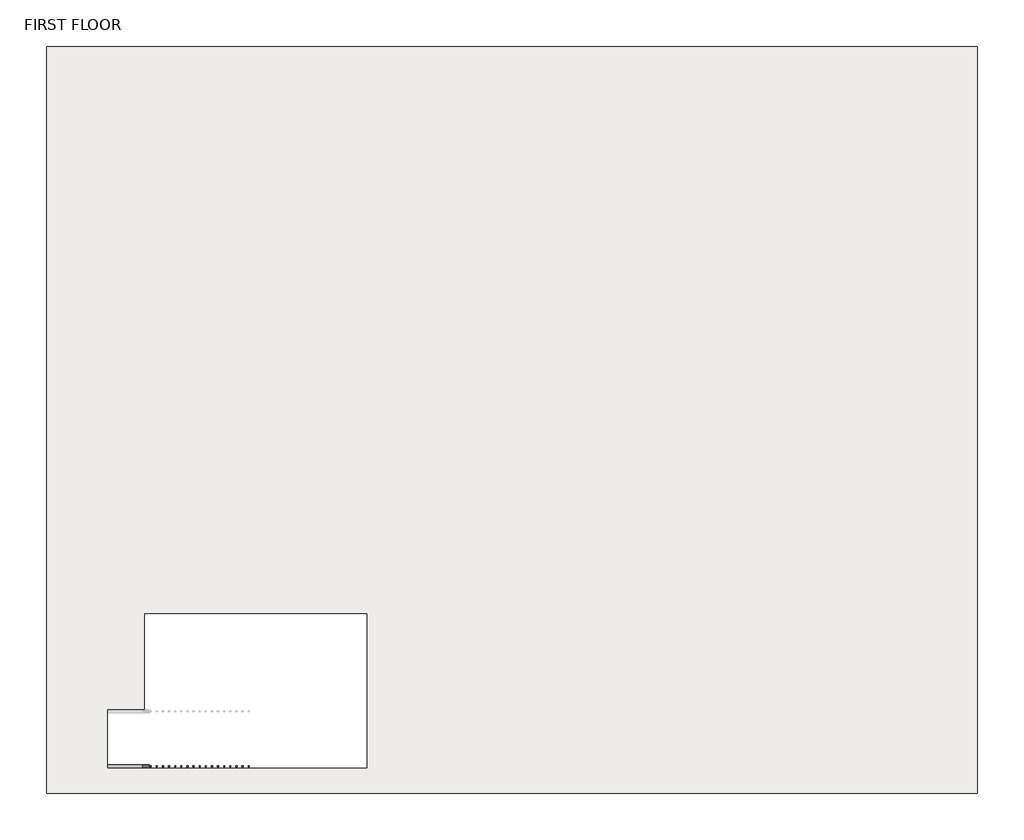
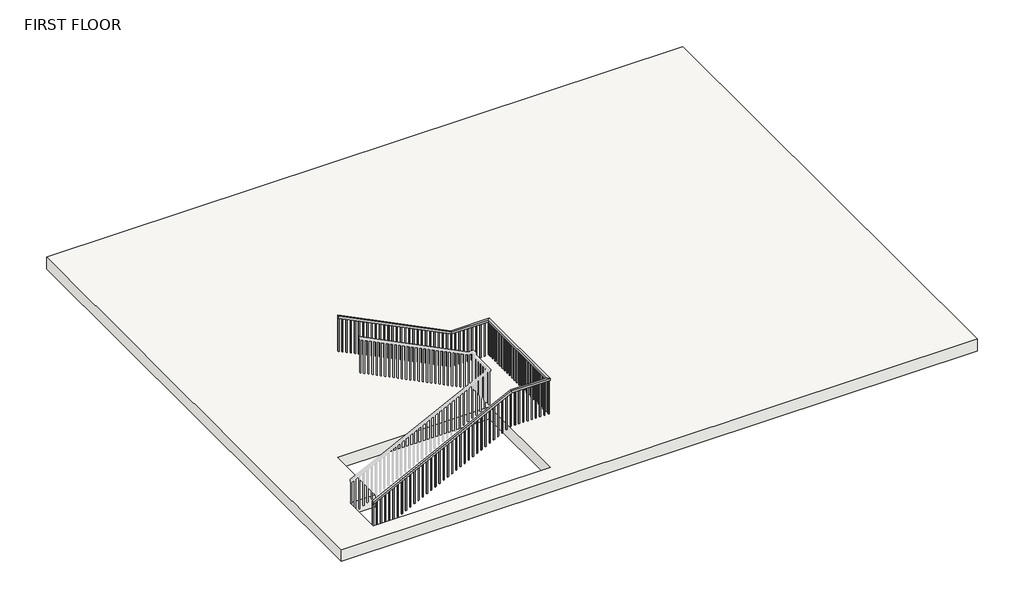
# One storey, part 1 of 2: 1 railing, 1 slab.
"""IFC4 building model written with IfcOpenShell, lengths in millimetres."""

from ifc_helpers import new_model, si_unit, frame, origin, place, context, project, spatial, polyline, outline, extrude, faceted_brep, element, save

model = new_model("IFC4")

# Units and contexts
model_context = context("Model", 3, world=origin())
ifc_project = project(units=[si_unit("LENGTHUNIT", "METRE", prefix="MILLI")], contexts=[model_context])

# Site, building, storey
site = spatial("IfcSite", under=ifc_project)
building = spatial("IfcBuilding", under=site)
storey = spatial("IfcBuildingStorey", under=building, Name="FIRST FLOOR", Elevation=3048.0)

# Railing
placement = place(None, origin())
element("IfcRailing", 1, ObjectType="Handrail - Rectangular", at=placement, inside=storey, context=model_context, shape_type="SolidModel", body=[
    faceted_brep([(-8362.2800418, -5370.1090076, 3962.4), (-8362.2800418, -5370.1090076, 3905.6038734), (-8362.2800418, -5420.9090076, 3905.6038734), (-8362.2800418, -5420.9090076, 3962.4), (-5009.4800418, -5370.1090076, 5638.8), (-4997.4877885, -5370.1090076, 5588.0), (-4997.4877885, -5420.9090076, 5588.0), (-5009.4800418, -5420.9090076, 5638.8), (-4120.4800418, -5370.1090076, 5638.8), (-4120.4800418, -5370.1090076, 5588.0), (-4069.6800418, -5420.9090076, 5588.0), (-4069.6800418, -5420.9090076, 5638.8), (-4120.4800418, -2917.1346494, 5638.8), (-4120.4800418, -2917.1346494, 5588.0), (-4069.6800418, -2866.3346494, 5588.0), (-4069.6800418, -2866.3346494, 5638.8), (-5009.4800418, -2917.1346494, 5638.8), (-5021.472295, -2917.1346494, 5588.0), (-5021.472295, -2866.3346494, 5588.0), (-5009.4800418, -2866.3346494, 5638.8), (-7752.6800418, -2917.1346494, 7010.4), (-7752.6800418, -2866.3346494, 7010.4), (-7752.6800418, -2866.3346494, 6953.6038734), (-7752.6800418, -2917.1346494, 6953.6038734)], [[[0, 1, 2, 3]], [[1, 0, 4, 5]], [[2, 1, 5, 6]], [[3, 2, 6, 7]], [[0, 3, 7, 4]], [[5, 4, 8, 9]], [[6, 5, 9, 10]], [[7, 6, 10, 11]], [[4, 7, 11, 8]], [[9, 8, 12, 13]], [[10, 9, 13, 14]], [[11, 10, 14, 15]], [[8, 11, 15, 12]], [[13, 12, 16, 17]], [[14, 13, 17, 18]], [[15, 14, 18, 19]], [[12, 15, 19, 16]], [[20, 21, 22, 23]], [[17, 16, 20, 23]], [[18, 17, 23, 22]], [[19, 18, 22, 21]], [[16, 19, 21, 20]]]),
    extrude(outline(polyline([(6907.5663734, -7660.6050418), (6049.9625, -7660.6050418), (6040.4375, -7641.5550418), (6898.0413734, -7641.5550418), (6907.5663734, -7660.6050418)])), frame((0.0, -2901.2596494, 0.0), z_axis=(0.0, 1.0, 0.0), x_axis=(0.0, 0.0, 1.0)), (0.0, 0.0, 1.0), 19.05),
    extrude(outline(polyline([(6856.7663734, -7559.0050418), (5999.1625, -7559.0050418), (5989.6375, -7539.9550418), (6847.2413734, -7539.9550418), (6856.7663734, -7559.0050418)])), frame((0.0, -2901.2596494, 0.0), z_axis=(0.0, 1.0, 0.0), x_axis=(0.0, 0.0, 1.0)), (0.0, 0.0, 1.0), 19.05),
    extrude(outline(polyline([(6805.9663734, -7457.4050418), (5948.3625, -7457.4050418), (5938.8375, -7438.3550418), (6796.4413734, -7438.3550418), (6805.9663734, -7457.4050418)])), frame((0.0, -2901.2596494, 0.0), z_axis=(0.0, 1.0, 0.0), x_axis=(0.0, 0.0, 1.0)), (0.0, 0.0, 1.0), 19.05),
    extrude(outline(polyline([(6755.1663734, -7355.8050418), (5897.5625, -7355.8050418), (5888.0375, -7336.7550418), (6745.6413734, -7336.7550418), (6755.1663734, -7355.8050418)])), frame((0.0, -2901.2596494, 0.0), z_axis=(0.0, 1.0, 0.0), x_axis=(0.0, 0.0, 1.0)), (0.0, 0.0, 1.0), 19.05),
    extrude(outline(polyline([(6704.3663734, -7254.2050418), (5846.7625, -7254.2050418), (5837.2375, -7235.1550418), (6694.8413734, -7235.1550418), (6704.3663734, -7254.2050418)])), frame((0.0, -2901.2596494, 0.0), z_axis=(0.0, 1.0, 0.0), x_axis=(0.0, 0.0, 1.0)), (0.0, 0.0, 1.0), 19.05),
    extrude(outline(polyline([(6653.5663734, -7152.6050418), (5795.9625, -7152.6050418), (5786.4375, -7133.5550418), (6644.0413734, -7133.5550418), (6653.5663734, -7152.6050418)])), frame((0.0, -2901.2596494, 0.0), z_axis=(0.0, 1.0, 0.0), x_axis=(0.0, 0.0, 1.0)), (0.0, 0.0, 1.0), 19.05),
    extrude(outline(polyline([(6602.7663734, -7051.0050418), (5745.1625, -7051.0050418), (5735.6375, -7031.9550418), (6593.2413734, -7031.9550418), (6602.7663734, -7051.0050418)])), frame((0.0, -2901.2596494, 0.0), z_axis=(0.0, 1.0, 0.0), x_axis=(0.0, 0.0, 1.0)), (0.0, 0.0, 1.0), 19.05),
    extrude(outline(polyline([(6551.9663734, -6949.4050418), (5694.3625, -6949.4050418), (5684.8375, -6930.3550418), (6542.4413734, -6930.3550418), (6551.9663734, -6949.4050418)])), frame((0.0, -2901.2596494, 0.0), z_axis=(0.0, 1.0, 0.0), x_axis=(0.0, 0.0, 1.0)), (0.0, 0.0, 1.0), 19.05),
    extrude(outline(polyline([(6501.1663734, -6847.8050418), (5643.5625, -6847.8050418), (5634.0375, -6828.7550418), (6491.6413734, -6828.7550418), (6501.1663734, -6847.8050418)])), frame((0.0, -2901.2596494, 0.0), z_axis=(0.0, 1.0, 0.0), x_axis=(0.0, 0.0, 1.0)), (0.0, 0.0, 1.0), 19.05),
    extrude(outline(polyline([(6450.3663734, -6746.2050418), (5592.7625, -6746.2050418), (5583.2375, -6727.1550418), (6440.8413734, -6727.1550418), (6450.3663734, -6746.2050418)])), frame((0.0, -2901.2596494, 0.0), z_axis=(0.0, 1.0, 0.0), x_axis=(0.0, 0.0, 1.0)), (0.0, 0.0, 1.0), 19.05),
    extrude(outline(polyline([(6399.5663734, -6644.6050418), (5541.9625, -6644.6050418), (5532.4375, -6625.5550418), (6390.0413734, -6625.5550418), (6399.5663734, -6644.6050418)])), frame((0.0, -2901.2596494, 0.0), z_axis=(0.0, 1.0, 0.0), x_axis=(0.0, 0.0, 1.0)), (0.0, 0.0, 1.0), 19.05),
    extrude(outline(polyline([(6348.7663734, -6543.0050418), (5491.1625, -6543.0050418), (5481.6375, -6523.9550418), (6339.2413734, -6523.9550418), (6348.7663734, -6543.0050418)])), frame((0.0, -2901.2596494, 0.0), z_axis=(0.0, 1.0, 0.0), x_axis=(0.0, 0.0, 1.0)), (0.0, 0.0, 1.0), 19.05),
    extrude(outline(polyline([(6297.9663734, -6441.4050418), (5440.3625, -6441.4050418), (5430.8375, -6422.3550418), (6288.4413734, -6422.3550418), (6297.9663734, -6441.4050418)])), frame((0.0, -2901.2596494, 0.0), z_axis=(0.0, 1.0, 0.0), x_axis=(0.0, 0.0, 1.0)), (0.0, 0.0, 1.0), 19.05),
    extrude(outline(polyline([(6247.1663734, -6339.8050418), (5389.5625, -6339.8050418), (5380.0375, -6320.7550418), (6237.6413734, -6320.7550418), (6247.1663734, -6339.8050418)])), frame((0.0, -2901.2596494, 0.0), z_axis=(0.0, 1.0, 0.0), x_axis=(0.0, 0.0, 1.0)), (0.0, 0.0, 1.0), 19.05),
    extrude(outline(polyline([(6196.3663734, -6238.2050418), (5338.7625, -6238.2050418), (5329.2375, -6219.1550418), (6186.8413734, -6219.1550418), (6196.3663734, -6238.2050418)])), frame((0.0, -2901.2596494, 0.0), z_axis=(0.0, 1.0, 0.0), x_axis=(0.0, 0.0, 1.0)), (0.0, 0.0, 1.0), 19.05),
    extrude(outline(polyline([(6145.5663734, -6136.6050418), (5287.9625, -6136.6050418), (5278.4375, -6117.5550418), (6136.0413734, -6117.5550418), (6145.5663734, -6136.6050418)])), frame((0.0, -2901.2596494, 0.0), z_axis=(0.0, 1.0, 0.0), x_axis=(0.0, 0.0, 1.0)), (0.0, 0.0, 1.0), 19.05),
    extrude(outline(polyline([(6094.7663734, -6035.0050418), (5237.1625, -6035.0050418), (5227.6375, -6015.9550418), (6085.2413734, -6015.9550418), (6094.7663734, -6035.0050418)])), frame((0.0, -2901.2596494, 0.0), z_axis=(0.0, 1.0, 0.0), x_axis=(0.0, 0.0, 1.0)), (0.0, 0.0, 1.0), 19.05),
    extrude(outline(polyline([(6043.9663734, -5933.4050418), (5186.3625, -5933.4050418), (5176.8375, -5914.3550418), (6034.4413734, -5914.3550418), (6043.9663734, -5933.4050418)])), frame((0.0, -2901.2596494, 0.0), z_axis=(0.0, 1.0, 0.0), x_axis=(0.0, 0.0, 1.0)), (0.0, 0.0, 1.0), 19.05),
    extrude(outline(polyline([(5993.1663734, -5831.8050418), (5135.5625, -5831.8050418), (5126.0375, -5812.7550418), (5983.6413734, -5812.7550418), (5993.1663734, -5831.8050418)])), frame((0.0, -2901.2596494, 0.0), z_axis=(0.0, 1.0, 0.0), x_axis=(0.0, 0.0, 1.0)), (0.0, 0.0, 1.0), 19.05),
    extrude(outline(polyline([(5942.3663734, -5730.2050418), (5084.7625, -5730.2050418), (5075.2375, -5711.1550418), (5932.8413734, -5711.1550418), (5942.3663734, -5730.2050418)])), frame((0.0, -2901.2596494, 0.0), z_axis=(0.0, 1.0, 0.0), x_axis=(0.0, 0.0, 1.0)), (0.0, 0.0, 1.0), 19.05),
    extrude(outline(polyline([(5891.5663734, -5628.6050418), (5033.9625, -5628.6050418), (5024.4375, -5609.5550418), (5882.0413734, -5609.5550418), (5891.5663734, -5628.6050418)])), frame((0.0, -2901.2596494, 0.0), z_axis=(0.0, 1.0, 0.0), x_axis=(0.0, 0.0, 1.0)), (0.0, 0.0, 1.0), 19.05),
    extrude(outline(polyline([(5840.7663734, -5527.0050418), (4983.1625, -5527.0050418), (4973.6375, -5507.9550418), (5831.2413734, -5507.9550418), (5840.7663734, -5527.0050418)])), frame((0.0, -2901.2596494, 0.0), z_axis=(0.0, 1.0, 0.0), x_axis=(0.0, 0.0, 1.0)), (0.0, 0.0, 1.0), 19.05),
    extrude(outline(polyline([(5789.9663734, -5425.4050418), (4932.3625, -5425.4050418), (4922.8375, -5406.3550418), (5780.4413734, -5406.3550418), (5789.9663734, -5425.4050418)])), frame((0.0, -2901.2596494, 0.0), z_axis=(0.0, 1.0, 0.0), x_axis=(0.0, 0.0, 1.0)), (0.0, 0.0, 1.0), 19.05),
    extrude(outline(polyline([(5739.1663734, -5323.8050418), (4881.5625, -5323.8050418), (4872.0375, -5304.7550418), (5729.6413734, -5304.7550418), (5739.1663734, -5323.8050418)])), frame((0.0, -2901.2596494, 0.0), z_axis=(0.0, 1.0, 0.0), x_axis=(0.0, 0.0, 1.0)), (0.0, 0.0, 1.0), 19.05),
    extrude(outline(polyline([(5688.3663734, -5222.2050418), (4830.7625, -5222.2050418), (4821.2375, -5203.1550418), (5678.8413734, -5203.1550418), (5688.3663734, -5222.2050418)])), frame((0.0, -2901.2596494, 0.0), z_axis=(0.0, 1.0, 0.0), x_axis=(0.0, 0.0, 1.0)), (0.0, 0.0, 1.0), 19.05),
    extrude(outline(polyline([(5637.5663734, -5120.6050418), (4779.9625, -5120.6050418), (4770.4375, -5101.5550418), (5628.0413734, -5101.5550418), (5637.5663734, -5120.6050418)])), frame((0.0, -2901.2596494, 0.0), z_axis=(0.0, 1.0, 0.0), x_axis=(0.0, 0.0, 1.0)), (0.0, 0.0, 1.0), 19.05),
    extrude(outline(polyline([(-4898.3550418, -2901.2596494), (-4917.4050418, -2901.2596494), (-4917.4050418, -2882.2096494), (-4898.3550418, -2882.2096494), (-4898.3550418, -2901.2596494)])), frame((0.0, 0.0, 4724.4), z_axis=(0.0, 0.0, 1.0), x_axis=(1.0, 0.0, 0.0)), (0.0, 0.0, 1.0), 863.6),
    extrude(outline(polyline([(-4796.7550418, -2901.2596494), (-4815.8050418, -2901.2596494), (-4815.8050418, -2882.2096494), (-4796.7550418, -2882.2096494), (-4796.7550418, -2901.2596494)])), frame((0.0, 0.0, 4724.4), z_axis=(0.0, 0.0, 1.0), x_axis=(1.0, 0.0, 0.0)), (0.0, 0.0, 1.0), 863.6),
    extrude(outline(polyline([(-4695.1550418, -2901.2596494), (-4714.2050418, -2901.2596494), (-4714.2050418, -2882.2096494), (-4695.1550418, -2882.2096494), (-4695.1550418, -2901.2596494)])), frame((0.0, 0.0, 4724.4), z_axis=(0.0, 0.0, 1.0), x_axis=(1.0, 0.0, 0.0)), (0.0, 0.0, 1.0), 863.6),
    extrude(outline(polyline([(-4593.5550418, -2901.2596494), (-4612.6050418, -2901.2596494), (-4612.6050418, -2882.2096494), (-4593.5550418, -2882.2096494), (-4593.5550418, -2901.2596494)])), frame((0.0, 0.0, 4724.4), z_axis=(0.0, 0.0, 1.0), x_axis=(1.0, 0.0, 0.0)), (0.0, 0.0, 1.0), 863.6),
    extrude(outline(polyline([(-4491.9550418, -2901.2596494), (-4511.0050418, -2901.2596494), (-4511.0050418, -2882.2096494), (-4491.9550418, -2882.2096494), (-4491.9550418, -2901.2596494)])), frame((0.0, 0.0, 4724.4), z_axis=(0.0, 0.0, 1.0), x_axis=(1.0, 0.0, 0.0)), (0.0, 0.0, 1.0), 863.6),
    extrude(outline(polyline([(-4390.3550418, -2901.2596494), (-4409.4050418, -2901.2596494), (-4409.4050418, -2882.2096494), (-4390.3550418, -2882.2096494), (-4390.3550418, -2901.2596494)])), frame((0.0, 0.0, 4724.4), z_axis=(0.0, 0.0, 1.0), x_axis=(1.0, 0.0, 0.0)), (0.0, 0.0, 1.0), 863.6),
    extrude(outline(polyline([(-4288.7550418, -2901.2596494), (-4307.8050418, -2901.2596494), (-4307.8050418, -2882.2096494), (-4288.7550418, -2882.2096494), (-4288.7550418, -2901.2596494)])), frame((0.0, 0.0, 4724.4), z_axis=(0.0, 0.0, 1.0), x_axis=(1.0, 0.0, 0.0)), (0.0, 0.0, 1.0), 863.6),
    extrude(outline(polyline([(-4187.1550418, -2901.2596494), (-4206.2050418, -2901.2596494), (-4206.2050418, -2882.2096494), (-4187.1550418, -2882.2096494), (-4187.1550418, -2901.2596494)])), frame((0.0, 0.0, 4724.4), z_axis=(0.0, 0.0, 1.0), x_axis=(1.0, 0.0, 0.0)), (0.0, 0.0, 1.0), 863.6),
    extrude(outline(polyline([(-4104.6050418, -2966.6340076), (-4104.6050418, -2947.5840076), (-4085.5550418, -2947.5840076), (-4085.5550418, -2966.6340076), (-4104.6050418, -2966.6340076)])), frame((0.0, 0.0, 4724.4), z_axis=(0.0, 0.0, 1.0), x_axis=(1.0, 0.0, 0.0)), (0.0, 0.0, 1.0), 863.6),
    extrude(outline(polyline([(-4104.6050418, -3068.2340076), (-4104.6050418, -3049.1840076), (-4085.5550418, -3049.1840076), (-4085.5550418, -3068.2340076), (-4104.6050418, -3068.2340076)])), frame((0.0, 0.0, 4724.4), z_axis=(0.0, 0.0, 1.0), x_axis=(1.0, 0.0, 0.0)), (0.0, 0.0, 1.0), 863.6),
    extrude(outline(polyline([(-4104.6050418, -3169.8340076), (-4104.6050418, -3150.7840076), (-4085.5550418, -3150.7840076), (-4085.5550418, -3169.8340076), (-4104.6050418, -3169.8340076)])), frame((0.0, 0.0, 4724.4), z_axis=(0.0, 0.0, 1.0), x_axis=(1.0, 0.0, 0.0)), (0.0, 0.0, 1.0), 863.6),
    extrude(outline(polyline([(-4104.6050418, -3271.4340076), (-4104.6050418, -3252.3840076), (-4085.5550418, -3252.3840076), (-4085.5550418, -3271.4340076), (-4104.6050418, -3271.4340076)])), frame((0.0, 0.0, 4724.4), z_axis=(0.0, 0.0, 1.0), x_axis=(1.0, 0.0, 0.0)), (0.0, 0.0, 1.0), 863.6),
    extrude(outline(polyline([(-4104.6050418, -3373.0340076), (-4104.6050418, -3353.9840076), (-4085.5550418, -3353.9840076), (-4085.5550418, -3373.0340076), (-4104.6050418, -3373.0340076)])), frame((0.0, 0.0, 4724.4), z_axis=(0.0, 0.0, 1.0), x_axis=(1.0, 0.0, 0.0)), (0.0, 0.0, 1.0), 863.6),
    extrude(outline(polyline([(-4104.6050418, -3474.6340076), (-4104.6050418, -3455.5840076), (-4085.5550418, -3455.5840076), (-4085.5550418, -3474.6340076), (-4104.6050418, -3474.6340076)])), frame((0.0, 0.0, 4724.4), z_axis=(0.0, 0.0, 1.0), x_axis=(1.0, 0.0, 0.0)), (0.0, 0.0, 1.0), 863.6),
    extrude(outline(polyline([(-4104.6050418, -3576.2340076), (-4104.6050418, -3557.1840076), (-4085.5550418, -3557.1840076), (-4085.5550418, -3576.2340076), (-4104.6050418, -3576.2340076)])), frame((0.0, 0.0, 4724.4), z_axis=(0.0, 0.0, 1.0), x_axis=(1.0, 0.0, 0.0)), (0.0, 0.0, 1.0), 863.6),
    extrude(outline(polyline([(-4104.6050418, -3677.8340076), (-4104.6050418, -3658.7840076), (-4085.5550418, -3658.7840076), (-4085.5550418, -3677.8340076), (-4104.6050418, -3677.8340076)])), frame((0.0, 0.0, 4724.4), z_axis=(0.0, 0.0, 1.0), x_axis=(1.0, 0.0, 0.0)), (0.0, 0.0, 1.0), 863.6),
    extrude(outline(polyline([(-4104.6050418, -3779.4340076), (-4104.6050418, -3760.3840076), (-4085.5550418, -3760.3840076), (-4085.5550418, -3779.4340076), (-4104.6050418, -3779.4340076)])), frame((0.0, 0.0, 4724.4), z_axis=(0.0, 0.0, 1.0), x_axis=(1.0, 0.0, 0.0)), (0.0, 0.0, 1.0), 863.6),
    extrude(outline(polyline([(-4104.6050418, -3881.0340076), (-4104.6050418, -3861.9840076), (-4085.5550418, -3861.9840076), (-4085.5550418, -3881.0340076), (-4104.6050418, -3881.0340076)])), frame((0.0, 0.0, 4724.4), z_axis=(0.0, 0.0, 1.0), x_axis=(1.0, 0.0, 0.0)), (0.0, 0.0, 1.0), 863.6),
    extrude(outline(polyline([(-4104.6050418, -3982.6340076), (-4104.6050418, -3963.5840076), (-4085.5550418, -3963.5840076), (-4085.5550418, -3982.6340076), (-4104.6050418, -3982.6340076)])), frame((0.0, 0.0, 4724.4), z_axis=(0.0, 0.0, 1.0), x_axis=(1.0, 0.0, 0.0)), (0.0, 0.0, 1.0), 863.6),
    extrude(outline(polyline([(-4104.6050418, -4084.2340076), (-4104.6050418, -4065.1840076), (-4085.5550418, -4065.1840076), (-4085.5550418, -4084.2340076), (-4104.6050418, -4084.2340076)])), frame((0.0, 0.0, 4724.4), z_axis=(0.0, 0.0, 1.0), x_axis=(1.0, 0.0, 0.0)), (0.0, 0.0, 1.0), 863.6),
    extrude(outline(polyline([(-4104.6050418, -4185.8340076), (-4104.6050418, -4166.7840076), (-4085.5550418, -4166.7840076), (-4085.5550418, -4185.8340076), (-4104.6050418, -4185.8340076)])), frame((0.0, 0.0, 4724.4), z_axis=(0.0, 0.0, 1.0), x_axis=(1.0, 0.0, 0.0)), (0.0, 0.0, 1.0), 863.6),
    extrude(outline(polyline([(-4104.6050418, -4287.4340076), (-4104.6050418, -4268.3840076), (-4085.5550418, -4268.3840076), (-4085.5550418, -4287.4340076), (-4104.6050418, -4287.4340076)])), frame((0.0, 0.0, 4724.4), z_axis=(0.0, 0.0, 1.0), x_axis=(1.0, 0.0, 0.0)), (0.0, 0.0, 1.0), 863.6),
    extrude(outline(polyline([(-4104.6050418, -4389.0340076), (-4104.6050418, -4369.9840076), (-4085.5550418, -4369.9840076), (-4085.5550418, -4389.0340076), (-4104.6050418, -4389.0340076)])), frame((0.0, 0.0, 4724.4), z_axis=(0.0, 0.0, 1.0), x_axis=(1.0, 0.0, 0.0)), (0.0, 0.0, 1.0), 863.6),
    extrude(outline(polyline([(-4104.6050418, -4490.6340076), (-4104.6050418, -4471.5840076), (-4085.5550418, -4471.5840076), (-4085.5550418, -4490.6340076), (-4104.6050418, -4490.6340076)])), frame((0.0, 0.0, 4724.4), z_axis=(0.0, 0.0, 1.0), x_axis=(1.0, 0.0, 0.0)), (0.0, 0.0, 1.0), 863.6),
    extrude(outline(polyline([(-4104.6050418, -4592.2340076), (-4104.6050418, -4573.1840076), (-4085.5550418, -4573.1840076), (-4085.5550418, -4592.2340076), (-4104.6050418, -4592.2340076)])), frame((0.0, 0.0, 4724.4), z_axis=(0.0, 0.0, 1.0), x_axis=(1.0, 0.0, 0.0)), (0.0, 0.0, 1.0), 863.6),
    extrude(outline(polyline([(-4104.6050418, -4693.8340076), (-4104.6050418, -4674.7840076), (-4085.5550418, -4674.7840076), (-4085.5550418, -4693.8340076), (-4104.6050418, -4693.8340076)])), frame((0.0, 0.0, 4724.4), z_axis=(0.0, 0.0, 1.0), x_axis=(1.0, 0.0, 0.0)), (0.0, 0.0, 1.0), 863.6),
    extrude(outline(polyline([(-4104.6050418, -4795.4340076), (-4104.6050418, -4776.3840076), (-4085.5550418, -4776.3840076), (-4085.5550418, -4795.4340076), (-4104.6050418, -4795.4340076)])), frame((0.0, 0.0, 4724.4), z_axis=(0.0, 0.0, 1.0), x_axis=(1.0, 0.0, 0.0)), (0.0, 0.0, 1.0), 863.6),
    extrude(outline(polyline([(-4104.6050418, -4897.0340076), (-4104.6050418, -4877.9840076), (-4085.5550418, -4877.9840076), (-4085.5550418, -4897.0340076), (-4104.6050418, -4897.0340076)])), frame((0.0, 0.0, 4724.4), z_axis=(0.0, 0.0, 1.0), x_axis=(1.0, 0.0, 0.0)), (0.0, 0.0, 1.0), 863.6),
    extrude(outline(polyline([(-4104.6050418, -4998.6340076), (-4104.6050418, -4979.5840076), (-4085.5550418, -4979.5840076), (-4085.5550418, -4998.6340076), (-4104.6050418, -4998.6340076)])), frame((0.0, 0.0, 4724.4), z_axis=(0.0, 0.0, 1.0), x_axis=(1.0, 0.0, 0.0)), (0.0, 0.0, 1.0), 863.6),
    extrude(outline(polyline([(-4104.6050418, -5100.2340076), (-4104.6050418, -5081.1840076), (-4085.5550418, -5081.1840076), (-4085.5550418, -5100.2340076), (-4104.6050418, -5100.2340076)])), frame((0.0, 0.0, 4724.4), z_axis=(0.0, 0.0, 1.0), x_axis=(1.0, 0.0, 0.0)), (0.0, 0.0, 1.0), 863.6),
    extrude(outline(polyline([(-4104.6050418, -5201.8340076), (-4104.6050418, -5182.7840076), (-4085.5550418, -5182.7840076), (-4085.5550418, -5201.8340076), (-4104.6050418, -5201.8340076)])), frame((0.0, 0.0, 4724.4), z_axis=(0.0, 0.0, 1.0), x_axis=(1.0, 0.0, 0.0)), (0.0, 0.0, 1.0), 863.6),
    extrude(outline(polyline([(-4104.6050418, -5303.4340076), (-4104.6050418, -5284.3840076), (-4085.5550418, -5284.3840076), (-4085.5550418, -5303.4340076), (-4104.6050418, -5303.4340076)])), frame((0.0, 0.0, 4724.4), z_axis=(0.0, 0.0, 1.0), x_axis=(1.0, 0.0, 0.0)), (0.0, 0.0, 1.0), 863.6),
    extrude(outline(polyline([(-4206.2050418, -5385.9840076), (-4187.1550418, -5385.9840076), (-4187.1550418, -5405.0340076), (-4206.2050418, -5405.0340076), (-4206.2050418, -5385.9840076)])), frame((0.0, 0.0, 4724.4), z_axis=(0.0, 0.0, 1.0), x_axis=(1.0, 0.0, 0.0)), (0.0, 0.0, 1.0), 863.6),
    extrude(outline(polyline([(-4307.8050418, -5385.9840076), (-4288.7550418, -5385.9840076), (-4288.7550418, -5405.0340076), (-4307.8050418, -5405.0340076), (-4307.8050418, -5385.9840076)])), frame((0.0, 0.0, 4724.4), z_axis=(0.0, 0.0, 1.0), x_axis=(1.0, 0.0, 0.0)), (0.0, 0.0, 1.0), 863.6),
    extrude(outline(polyline([(-4409.4050418, -5385.9840076), (-4390.3550418, -5385.9840076), (-4390.3550418, -5405.0340076), (-4409.4050418, -5405.0340076), (-4409.4050418, -5385.9840076)])), frame((0.0, 0.0, 4724.4), z_axis=(0.0, 0.0, 1.0), x_axis=(1.0, 0.0, 0.0)), (0.0, 0.0, 1.0), 863.6),
    extrude(outline(polyline([(-4511.0050418, -5385.9840076), (-4491.9550418, -5385.9840076), (-4491.9550418, -5405.0340076), (-4511.0050418, -5405.0340076), (-4511.0050418, -5385.9840076)])), frame((0.0, 0.0, 4724.4), z_axis=(0.0, 0.0, 1.0), x_axis=(1.0, 0.0, 0.0)), (0.0, 0.0, 1.0), 863.6),
    extrude(outline(polyline([(-4612.6050418, -5385.9840076), (-4593.5550418, -5385.9840076), (-4593.5550418, -5405.0340076), (-4612.6050418, -5405.0340076), (-4612.6050418, -5385.9840076)])), frame((0.0, 0.0, 4724.4), z_axis=(0.0, 0.0, 1.0), x_axis=(1.0, 0.0, 0.0)), (0.0, 0.0, 1.0), 863.6),
    extrude(outline(polyline([(-4714.2050418, -5385.9840076), (-4695.1550418, -5385.9840076), (-4695.1550418, -5405.0340076), (-4714.2050418, -5405.0340076), (-4714.2050418, -5385.9840076)])), frame((0.0, 0.0, 4724.4), z_axis=(0.0, 0.0, 1.0), x_axis=(1.0, 0.0, 0.0)), (0.0, 0.0, 1.0), 863.6),
    extrude(outline(polyline([(-4815.8050418, -5385.9840076), (-4796.7550418, -5385.9840076), (-4796.7550418, -5405.0340076), (-4815.8050418, -5405.0340076), (-4815.8050418, -5385.9840076)])), frame((0.0, 0.0, 4724.4), z_axis=(0.0, 0.0, 1.0), x_axis=(1.0, 0.0, 0.0)), (0.0, 0.0, 1.0), 863.6),
    extrude(outline(polyline([(-4917.4050418, -5385.9840076), (-4898.3550418, -5385.9840076), (-4898.3550418, -5405.0340076), (-4917.4050418, -5405.0340076), (-4917.4050418, -5385.9840076)])), frame((0.0, 0.0, 4724.4), z_axis=(0.0, 0.0, 1.0), x_axis=(1.0, 0.0, 0.0)), (0.0, 0.0, 1.0), 863.6),
    extrude(outline(polyline([(5526.4413734, -5120.6050418), (4668.8375, -5120.6050418), (4678.3625, -5101.5550418), (5535.9663734, -5101.5550418), (5526.4413734, -5120.6050418)])), frame((0.0, -5405.0340076, 0.0), z_axis=(0.0, 1.0, 0.0), x_axis=(0.0, 0.0, 1.0)), (0.0, 0.0, 1.0), 19.05),
    extrude(outline(polyline([(5475.6413734, -5222.2050418), (4618.0375, -5222.2050418), (4627.5625, -5203.1550418), (5485.1663734, -5203.1550418), (5475.6413734, -5222.2050418)])), frame((0.0, -5405.0340076, 0.0), z_axis=(0.0, 1.0, 0.0), x_axis=(0.0, 0.0, 1.0)), (0.0, 0.0, 1.0), 19.05),
    extrude(outline(polyline([(5424.8413734, -5323.8050418), (4567.2375, -5323.8050418), (4576.7625, -5304.7550418), (5434.3663734, -5304.7550418), (5424.8413734, -5323.8050418)])), frame((0.0, -5405.0340076, 0.0), z_axis=(0.0, 1.0, 0.0), x_axis=(0.0, 0.0, 1.0)), (0.0, 0.0, 1.0), 19.05),
    extrude(outline(polyline([(5374.0413734, -5425.4050418), (4516.4375, -5425.4050418), (4525.9625, -5406.3550418), (5383.5663734, -5406.3550418), (5374.0413734, -5425.4050418)])), frame((0.0, -5405.0340076, 0.0), z_axis=(0.0, 1.0, 0.0), x_axis=(0.0, 0.0, 1.0)), (0.0, 0.0, 1.0), 19.05),
    extrude(outline(polyline([(5323.2413734, -5527.0050418), (4465.6375, -5527.0050418), (4475.1625, -5507.9550418), (5332.7663734, -5507.9550418), (5323.2413734, -5527.0050418)])), frame((0.0, -5405.0340076, 0.0), z_axis=(0.0, 1.0, 0.0), x_axis=(0.0, 0.0, 1.0)), (0.0, 0.0, 1.0), 19.05),
    extrude(outline(polyline([(5272.4413734, -5628.6050418), (4414.8375, -5628.6050418), (4424.3625, -5609.5550418), (5281.9663734, -5609.5550418), (5272.4413734, -5628.6050418)])), frame((0.0, -5405.0340076, 0.0), z_axis=(0.0, 1.0, 0.0), x_axis=(0.0, 0.0, 1.0)), (0.0, 0.0, 1.0), 19.05),
    extrude(outline(polyline([(5221.6413734, -5730.2050418), (4364.0375, -5730.2050418), (4373.5625, -5711.1550418), (5231.1663734, -5711.1550418), (5221.6413734, -5730.2050418)])), frame((0.0, -5405.0340076, 0.0), z_axis=(0.0, 1.0, 0.0), x_axis=(0.0, 0.0, 1.0)), (0.0, 0.0, 1.0), 19.05),
    extrude(outline(polyline([(5170.8413734, -5831.8050418), (4313.2375, -5831.8050418), (4322.7625, -5812.7550418), (5180.3663734, -5812.7550418), (5170.8413734, -5831.8050418)])), frame((0.0, -5405.0340076, 0.0), z_axis=(0.0, 1.0, 0.0), x_axis=(0.0, 0.0, 1.0)), (0.0, 0.0, 1.0), 19.05),
    extrude(outline(polyline([(5120.0413734, -5933.4050418), (4262.4375, -5933.4050418), (4271.9625, -5914.3550418), (5129.5663734, -5914.3550418), (5120.0413734, -5933.4050418)])), frame((0.0, -5405.0340076, 0.0), z_axis=(0.0, 1.0, 0.0), x_axis=(0.0, 0.0, 1.0)), (0.0, 0.0, 1.0), 19.05),
    extrude(outline(polyline([(5069.2413734, -6035.0050418), (4211.6375, -6035.0050418), (4221.1625, -6015.9550418), (5078.7663734, -6015.9550418), (5069.2413734, -6035.0050418)])), frame((0.0, -5405.0340076, 0.0), z_axis=(0.0, 1.0, 0.0), x_axis=(0.0, 0.0, 1.0)), (0.0, 0.0, 1.0), 19.05),
    extrude(outline(polyline([(5018.4413734, -6136.6050418), (4160.8375, -6136.6050418), (4170.3625, -6117.5550418), (5027.9663734, -6117.5550418), (5018.4413734, -6136.6050418)])), frame((0.0, -5405.0340076, 0.0), z_axis=(0.0, 1.0, 0.0), x_axis=(0.0, 0.0, 1.0)), (0.0, 0.0, 1.0), 19.05),
    extrude(outline(polyline([(4967.6413734, -6238.2050418), (4110.0375, -6238.2050418), (4119.5625, -6219.1550418), (4977.1663734, -6219.1550418), (4967.6413734, -6238.2050418)])), frame((0.0, -5405.0340076, 0.0), z_axis=(0.0, 1.0, 0.0), x_axis=(0.0, 0.0, 1.0)), (0.0, 0.0, 1.0), 19.05),
    extrude(outline(polyline([(4916.8413734, -6339.8050418), (4059.2375, -6339.8050418), (4068.7625, -6320.7550418), (4926.3663734, -6320.7550418), (4916.8413734, -6339.8050418)])), frame((0.0, -5405.0340076, 0.0), z_axis=(0.0, 1.0, 0.0), x_axis=(0.0, 0.0, 1.0)), (0.0, 0.0, 1.0), 19.05),
    extrude(outline(polyline([(4866.0413734, -6441.4050418), (4008.4375, -6441.4050418), (4017.9625, -6422.3550418), (4875.5663734, -6422.3550418), (4866.0413734, -6441.4050418)])), frame((0.0, -5405.0340076, 0.0), z_axis=(0.0, 1.0, 0.0), x_axis=(0.0, 0.0, 1.0)), (0.0, 0.0, 1.0), 19.05),
    extrude(outline(polyline([(4815.2413734, -6543.0050418), (3957.6375, -6543.0050418), (3967.1625, -6523.9550418), (4824.7663734, -6523.9550418), (4815.2413734, -6543.0050418)])), frame((0.0, -5405.0340076, 0.0), z_axis=(0.0, 1.0, 0.0), x_axis=(0.0, 0.0, 1.0)), (0.0, 0.0, 1.0), 19.05),
    extrude(outline(polyline([(4764.4413734, -6644.6050418), (3906.8375, -6644.6050418), (3916.3625, -6625.5550418), (4773.9663734, -6625.5550418), (4764.4413734, -6644.6050418)])), frame((0.0, -5405.0340076, 0.0), z_axis=(0.0, 1.0, 0.0), x_axis=(0.0, 0.0, 1.0)), (0.0, 0.0, 1.0), 19.05),
    extrude(outline(polyline([(4713.6413734, -6746.2050418), (3856.0375, -6746.2050418), (3865.5625, -6727.1550418), (4723.1663734, -6727.1550418), (4713.6413734, -6746.2050418)])), frame((0.0, -5405.0340076, 0.0), z_axis=(0.0, 1.0, 0.0), x_axis=(0.0, 0.0, 1.0)), (0.0, 0.0, 1.0), 19.05),
    extrude(outline(polyline([(4662.8413734, -6847.8050418), (3805.2375, -6847.8050418), (3814.7625, -6828.7550418), (4672.3663734, -6828.7550418), (4662.8413734, -6847.8050418)])), frame((0.0, -5405.0340076, 0.0), z_axis=(0.0, 1.0, 0.0), x_axis=(0.0, 0.0, 1.0)), (0.0, 0.0, 1.0), 19.05),
    extrude(outline(polyline([(4612.0413734, -6949.4050418), (3754.4375, -6949.4050418), (3763.9625, -6930.3550418), (4621.5663734, -6930.3550418), (4612.0413734, -6949.4050418)])), frame((0.0, -5405.0340076, 0.0), z_axis=(0.0, 1.0, 0.0), x_axis=(0.0, 0.0, 1.0)), (0.0, 0.0, 1.0), 19.05),
    extrude(outline(polyline([(4561.2413734, -7051.0050418), (3703.6375, -7051.0050418), (3713.1625, -7031.9550418), (4570.7663734, -7031.9550418), (4561.2413734, -7051.0050418)])), frame((0.0, -5405.0340076, 0.0), z_axis=(0.0, 1.0, 0.0), x_axis=(0.0, 0.0, 1.0)), (0.0, 0.0, 1.0), 19.05),
    extrude(outline(polyline([(4510.4413734, -7152.6050418), (3652.8375, -7152.6050418), (3662.3625, -7133.5550418), (4519.9663734, -7133.5550418), (4510.4413734, -7152.6050418)])), frame((0.0, -5405.0340076, 0.0), z_axis=(0.0, 1.0, 0.0), x_axis=(0.0, 0.0, 1.0)), (0.0, 0.0, 1.0), 19.05),
    extrude(outline(polyline([(4459.6413734, -7254.2050418), (3602.0375, -7254.2050418), (3611.5625, -7235.1550418), (4469.1663734, -7235.1550418), (4459.6413734, -7254.2050418)])), frame((0.0, -5405.0340076, 0.0), z_axis=(0.0, 1.0, 0.0), x_axis=(0.0, 0.0, 1.0)), (0.0, 0.0, 1.0), 19.05),
    extrude(outline(polyline([(4408.8413734, -7355.8050418), (3551.2375, -7355.8050418), (3560.7625, -7336.7550418), (4418.3663734, -7336.7550418), (4408.8413734, -7355.8050418)])), frame((0.0, -5405.0340076, 0.0), z_axis=(0.0, 1.0, 0.0), x_axis=(0.0, 0.0, 1.0)), (0.0, 0.0, 1.0), 19.05),
    extrude(outline(polyline([(4358.0413734, -7457.4050418), (3500.4375, -7457.4050418), (3509.9625, -7438.3550418), (4367.5663734, -7438.3550418), (4358.0413734, -7457.4050418)])), frame((0.0, -5405.0340076, 0.0), z_axis=(0.0, 1.0, 0.0), x_axis=(0.0, 0.0, 1.0)), (0.0, 0.0, 1.0), 19.05),
    extrude(outline(polyline([(4307.2413734, -7559.0050418), (3449.6375, -7559.0050418), (3459.1625, -7539.9550418), (4316.7663734, -7539.9550418), (4307.2413734, -7559.0050418)])), frame((0.0, -5405.0340076, 0.0), z_axis=(0.0, 1.0, 0.0), x_axis=(0.0, 0.0, 1.0)), (0.0, 0.0, 1.0), 19.05),
    extrude(outline(polyline([(4256.4413734, -7660.6050418), (3398.8375, -7660.6050418), (3408.3625, -7641.5550418), (4265.9663734, -7641.5550418), (4256.4413734, -7660.6050418)])), frame((0.0, -5405.0340076, 0.0), z_axis=(0.0, 1.0, 0.0), x_axis=(0.0, 0.0, 1.0)), (0.0, 0.0, 1.0), 19.05),
    extrude(outline(polyline([(4205.6413734, -7762.2050418), (3348.0375, -7762.2050418), (3357.5625, -7743.1550418), (4215.1663734, -7743.1550418), (4205.6413734, -7762.2050418)])), frame((0.0, -5405.0340076, 0.0), z_axis=(0.0, 1.0, 0.0), x_axis=(0.0, 0.0, 1.0)), (0.0, 0.0, 1.0), 19.05),
    extrude(outline(polyline([(4154.8413734, -7863.8050418), (3297.2375, -7863.8050418), (3306.7625, -7844.7550418), (4164.3663734, -7844.7550418), (4154.8413734, -7863.8050418)])), frame((0.0, -5405.0340076, 0.0), z_axis=(0.0, 1.0, 0.0), x_axis=(0.0, 0.0, 1.0)), (0.0, 0.0, 1.0), 19.05),
    extrude(outline(polyline([(4104.0413734, -7965.4050418), (3246.4375, -7965.4050418), (3255.9625, -7946.3550418), (4113.5663734, -7946.3550418), (4104.0413734, -7965.4050418)])), frame((0.0, -5405.0340076, 0.0), z_axis=(0.0, 1.0, 0.0), x_axis=(0.0, 0.0, 1.0)), (0.0, 0.0, 1.0), 19.05),
    extrude(outline(polyline([(4053.2413734, -8067.0050418), (3195.6375, -8067.0050418), (3205.1625, -8047.9550418), (4062.7663734, -8047.9550418), (4053.2413734, -8067.0050418)])), frame((0.0, -5405.0340076, 0.0), z_axis=(0.0, 1.0, 0.0), x_axis=(0.0, 0.0, 1.0)), (0.0, 0.0, 1.0), 19.05),
    extrude(outline(polyline([(4002.4413734, -8168.6050418), (3144.8375, -8168.6050418), (3154.3625, -8149.5550418), (4011.9663734, -8149.5550418), (4002.4413734, -8168.6050418)])), frame((0.0, -5405.0340076, 0.0), z_axis=(0.0, 1.0, 0.0), x_axis=(0.0, 0.0, 1.0)), (0.0, 0.0, 1.0), 19.05),
    extrude(outline(polyline([(3951.6413734, -8270.2050418), (3094.0375, -8270.2050418), (3103.5625, -8251.1550418), (3961.1663734, -8251.1550418), (3951.6413734, -8270.2050418)])), frame((0.0, -5405.0340076, 0.0), z_axis=(0.0, 1.0, 0.0), x_axis=(0.0, 0.0, 1.0)), (0.0, 0.0, 1.0), 19.05),
    extrude(outline(polyline([(-4999.9550418, -2901.2596494), (-5019.0050418, -2901.2596494), (-5019.0050418, -2882.2096494), (-4999.9550418, -2882.2096494), (-4999.9550418, -2901.2596494)])), frame((0.0, 0.0, 4724.4), z_axis=(0.0, 0.0, 1.0), x_axis=(1.0, 0.0, 0.0)), (0.0, 0.0, 1.0), 863.6),
    extrude(outline(polyline([(-4104.6050418, -2901.2596494), (-4104.6050418, -2882.2096494), (-4085.5550418, -2882.2096494), (-4085.5550418, -2901.2596494), (-4104.6050418, -2901.2596494)])), frame((0.0, 0.0, 4724.4), z_axis=(0.0, 0.0, 1.0), x_axis=(1.0, 0.0, 0.0)), (0.0, 0.0, 1.0), 863.6),
    extrude(outline(polyline([(-4104.6050418, -5385.9840076), (-4085.5550418, -5385.9840076), (-4085.5550418, -5405.0340076), (-4104.6050418, -5405.0340076), (-4104.6050418, -5385.9840076)])), frame((0.0, 0.0, 4724.4), z_axis=(0.0, 0.0, 1.0), x_axis=(1.0, 0.0, 0.0)), (0.0, 0.0, 1.0), 863.6),
    extrude(outline(polyline([(5577.2413734, -5019.0050418), (4719.6375, -5019.0050418), (4729.1625, -4999.9550418), (5586.7663734, -4999.9550418), (5577.2413734, -5019.0050418)])), frame((0.0, -5405.0340076, 0.0), z_axis=(0.0, 1.0, 0.0), x_axis=(0.0, 0.0, 1.0)), (0.0, 0.0, 1.0), 19.05),
    extrude(outline(polyline([(6953.6038734, -7752.6800418), (6096.0, -7752.6800418), (6086.475, -7733.6300418), (6944.0788734, -7733.6300418), (6953.6038734, -7752.6800418)])), frame((0.0, -2901.2596494, 0.0), z_axis=(0.0, 1.0, 0.0), x_axis=(0.0, 0.0, 1.0)), (0.0, 0.0, 1.0), 19.05),
    extrude(outline(polyline([(3905.6038734, -8362.2800418), (3048.0, -8362.2800418), (3057.525, -8343.2300418), (3915.1288734, -8343.2300418), (3905.6038734, -8362.2800418)])), frame((0.0, -5405.0340076, 0.0), z_axis=(0.0, 1.0, 0.0), x_axis=(0.0, 0.0, 1.0)), (0.0, 0.0, 1.0), 19.05),
])

# Slab
element("IfcSlab", 2, ObjectType="Generic - 12\"", at=placement, inside=storey, context=model_context, shape_type="SweptSolid", body=[
    extrude(outline(polyline([(6064.2982466, 6554.3761968), (6064.2982466, -5840.8238032), (-9378.9017534, -5840.8238032), (-9378.9017534, 6554.3761968), (6064.2982466, 6554.3761968)]), holes=[polyline([(-7752.6800418, -2866.3346494), (-7752.6800418, -4455.7090076), (-8362.2800418, -4455.7090076), (-8362.2800418, -5420.9090076), (-4069.6800418, -5420.9090076), (-4069.6800418, -2866.3346494), (-7752.6800418, -2866.3346494)])]), frame((0.0, 0.0, 3048.0), z_axis=(0.0, 0.0, 1.0), x_axis=(1.0, 0.0, 0.0)), (0.0, 0.0, 1.0), 304.8),
])

save(model, "model.ifc")

# Revit data of these elements
# Type "Handrail - Rectangular"
#   Assembly Code = "C2010400"
#   built-in parameter 1008612 = 0.0416667 (stored number, unit not read)
#   built-in parameter 1008611 = 0.0416667 (stored number, unit not read)
#   built-in parameter 1008609 = 0.333333 (stored number, unit not read)
#   built-in parameter 1008604 = 0.166667 (stored number, unit not read)
#   built-in parameter 1008603 = 0.166667 (stored number, unit not read)
#   Railing Height = 3' - 0"
#   built-in parameter 1008630 = 2
#   built-in parameter 1008610 = 2
#   built-in parameter 1008618 = Baluster - Square : 3/4"
# Type "Generic - 12\""
#   Assembly Code = "B1010"
#   Function = 0
#   Layers, outside or top first: 1' - 0" no material (function 1)
# Element 1 (IfcRailing, "Handrail - Rectangular")
#   Phase Created = New Construction
# Element 2 (IfcSlab, "Generic - 12\"")
#   Height Offset From Level = 1' - 0"
#   Phase Created = New Construction
#   Materials on its faces: "Default Floor"
# Materials
#   "Default Floor": colour RGB 128 128 128, transparency 0, Cost = 0
